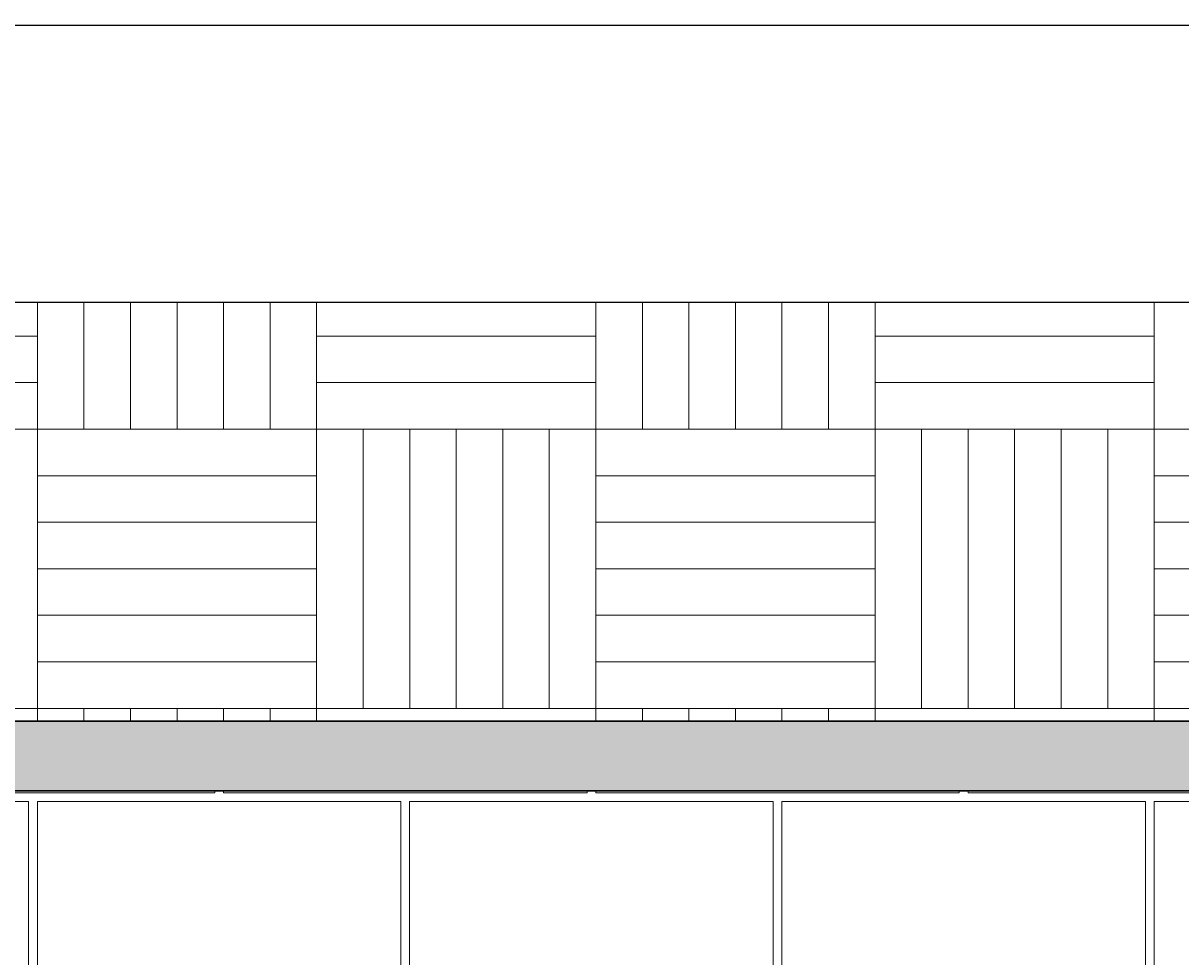
# Model space of a CAD drawing. Units: inches. Extents: x -128 to 854, y -395 to 398.
# Tile 59 of 61: x 467 to 567, y -248 to -167. Entities that reach past the tile are written whole.
import ezdxf

# ---------------------------------------------------------------- set-up
doc = ezdxf.new("R2010")
doc.units = ezdxf.units.IN
doc.header["$MEASUREMENT"] = 0
for name, color, linetype, lineweight in [('A-ANNO-DIMS', 2, 'Continuous', 18), ('A-ELEV', 3, 'Continuous', 25), ('A-ELEV-PATT', 8, 'Continuous', 13)]:
    doc.layers.add(name, color=color, linetype=linetype, lineweight=lineweight)
doc.styles.get("Standard").update_dxf_attribs({"font": 'arial.ttf'})
doc.dimstyles.get("Standard").update_dxf_attribs({"dimtxt": 0.18, "dimasz": 0.18, "dimexe": 0.18, "dimexo": 0.0625, "dimgap": 0.09, "dimtad": 0, "dimtih": 1, "dimtoh": 1, "dimdec": 1, "dimzin": 0, "dimdsep": 46, "dimlunit": 4, "dimtxsty": 'Standard', "dimcen": 0.09, "dimclrd": 1, "dimclre": 2, "dimclrt": 6, "dimadec": 0, "dimazin": 0, "dimtfac": 1, "dimtdec": 1, "dimtofl": 0, "dimtmove": 0, "dimatfit": 3, "dimfxl": 1, "dimtfill": 2, "dimtfillclr": 3, "dimtolj": 1, "dimtzin": 0, "dimarcsym": 0})

# ---------------------------------------------------------------- blocks, each defined once
blk = doc.blocks.new('*D133')
at = {"layer": 'A-ANNO-DIMS', "color": 2, "lineweight": -2, "transparency": 16777216}
for p, q in [((418.28, -191.414), (418.28, -167.496)), ((782.28, -191.414), (782.28, -167.496))]:
    blk.add_line(p, q, dxfattribs=at)
at = {"layer": 'A-ANNO-DIMS', "color": 1, "lineweight": -2, "transparency": 16777216}
for p, q in [((418.46, -167.676), (599.88, -167.676)), ((782.1, -167.676), (600.679, -167.676))]:
    blk.add_line(p, q, dxfattribs=at)
at = {"layer": 'A-ANNO-DIMS', "color": 1, "transparency": 16777216}
for points in [[(418.46, -167.646), (418.46, -167.706), (418.28, -167.676)], [(782.1, -167.646), (782.1, -167.706), (782.28, -167.676)]]:
    blk.add_solid(points, dxfattribs=at)
at = {"layer": 'Defpoints', "color": 0, "transparency": 16777216}
for p in [(782.28, -167.676), (418.28, -191.476), (782.28, -191.476)]:
    blk.add_point(p, dxfattribs=at)
at = {"layer": 'A-ANNO-DIMS', "color": 6, "transparency": 16777216, "insert": (600.28, -167.676), "char_height": 0.18, "attachment_point": 5, "bg_fill": 1, "box_fill_scale": 1.25, "bg_fill_color": 3, "bg_fill_transparency": 0}
blk.add_mtext('\\A1;30\'-4"', dxfattribs=at)

msp = doc.modelspace()

# ---------------------------------------------------------------- hatches: boundary and pattern name
at = {"layer": 'A-ELEV-PATT'}
h = msp.add_hatch(dxfattribs=at)
h.set_pattern_fill('AR-PARQ1', color=256, scale=2)
h.set_pattern_definition([(90, (468.407, -10.41), (-24, 24), [24, -24]), (90, (472.407, -10.41), (-24, 24), [24, -24]), (90, (476.407, -10.41), (-24, 24), [24, -24]), (90, (480.407, -10.41), (-24, 24), [24, -24]), (90, (484.407, -10.41), (-24, 24), [24, -24]), (90, (488.407, -10.41), (-24, 24), [24, -24]), (90, (492.407, -10.41), (-24, 24), [24, -24]), (0, (468.407, 13.59), (24, -24), [24, -24]), (0, (468.407, 17.59), (24, -24), [24, -24]), (0, (468.407, 21.59), (24, -24), [24, -24]), (0, (468.407, 25.59), (24, -24), [24, -24]), (0, (468.407, 29.59), (24, -24), [24, -24]), (0, (468.407, 33.59), (24, -24), [24, -24]), (0, (468.407, 37.59), (24, -24), [24, -24])])
h.paths.add_polyline_path([(782.28, -227.476), (782.28, -191.476), (418.28, -191.476), (418.28, -227.476)])
h = msp.add_hatch(color=256, dxfattribs=at)
h.dxf.hatch_style = 1
h.paths.add_polyline_path([(418.28, -227.476), (418.28, -233.476), (782.28, -233.476), (782.28, -227.476)])
h.paths.add_polyline_path([(492.252, -257.476), (492.252, -353.476), (551.307, -353.476), (551.307, -257.476)])
h.paths.add_polyline_path([(546.307, -262.476), (546.307, -348.476), (497.252, -348.476), (497.252, -262.476)], flags=16)
h = msp.add_hatch(dxfattribs=at)
h.set_pattern_fill('AR-B816C', color=256, scale=2)
h.set_pattern_definition([(0, (468.407, -10.41), (16, 16), [31.25, -0.75]), (0, (452.407, -9.66), (16, 16), [31.25, -0.75]), (90, (468.407, -10.41), (-16, 16), [-16.75, 15.25]), (90, (467.657, -10.41), (-16, 16), [-16.75, 15.25])])
h.paths.add_polyline_path([(418.28, -353.476), (492.252, -353.476), (492.252, -257.476), (551.307, -257.476), (551.307, -353.476), (782.28, -353.476), (782.28, -233.476), (418.28, -233.476)])
h.paths.add_polyline_path([(668.28, -257.476), (730.28, -257.476), (730.28, -305.476), (668.28, -305.476)], flags=16)
h.paths.add_polyline_path([(673.28, -300.476), (673.28, -262.476), (725.28, -262.476), (725.28, -300.476)], flags=0)

# ---------------------------------------------------------------- linework, layer by layer
at = {"layer": 'A-ELEV'}
for points in [[(418.28, -191.476), (782.28, -191.476), (782.28, -227.476), (418.28, -227.476)], [(418.28, -227.476), (782.28, -227.476), (782.28, -233.476), (418.28, -233.476)], [(418.28, -233.476), (782.28, -233.476), (782.28, -353.476), (418.28, -353.476)]]:
    msp.add_lwpolyline(points, close=True, dxfattribs=at)

# ---------------------------------------------------------------- dimensions: what is measured, and where the dimension line sits
at = {"layer": 'A-ANNO-DIMS'}
dim = msp.add_linear_dim(base=(782.28, -167.676), p1=(418.28, -191.476), p2=(782.28, -191.476), dimstyle='Standard', override={"dimdec": 1, "dimlfac": 1, "dimrnd": 0, "dimzin": 1, "dimdsep": 46, "dimlunit": 4, "dimfrac": 2}, dxfattribs=at)
dim.commit()
dim.dimension.update_dxf_attribs({"geometry": '*D133', "text_midpoint": (600.28, -167.676)})

doc.saveas('drawing.dxf')
